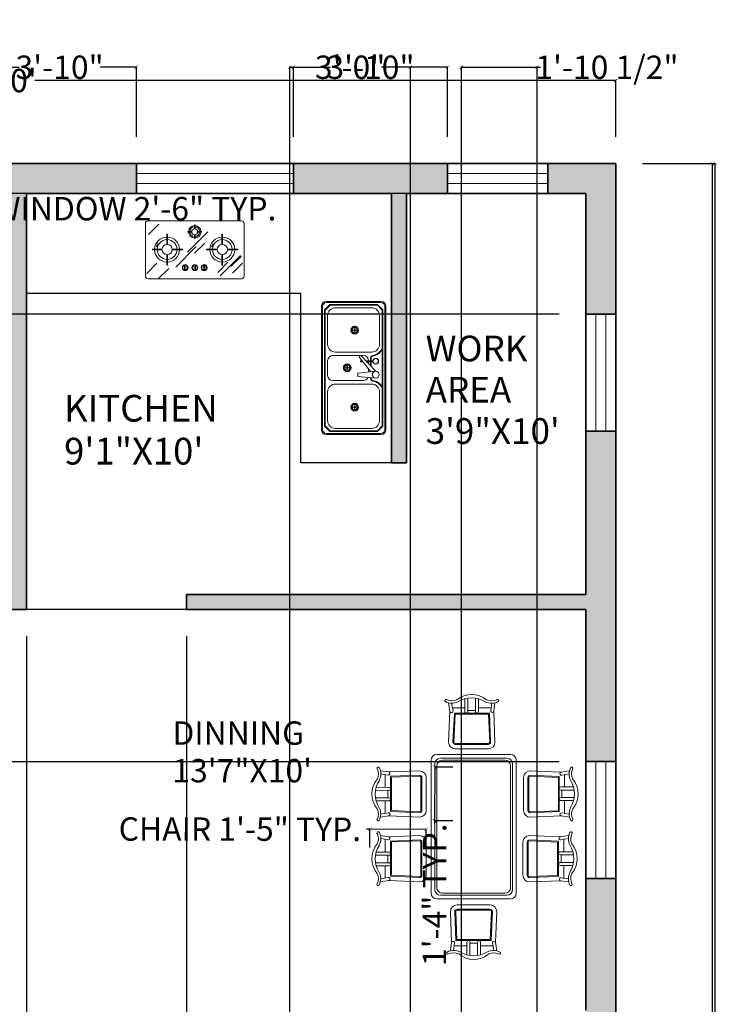
# Model space of a CAD drawing. Units: inches. Extents: x 98 to 545, y 56 to 703.
# Tile 4 of 4: x 324 to 537, y 408 to 703. Entities that reach past the tile are written whole.
import ezdxf

# ---------------------------------------------------------------- set-up
doc = ezdxf.new("R2010")
doc.units = ezdxf.units.IN
doc.header["$MEASUREMENT"] = 0
for name, color, linetype, lineweight in [('A-ANNO-DIMS', 2, 'Continuous', 18), ('A-AREA-IDEN', 7, 'Continuous', 25), ('A-EQPM', 8, 'Continuous', 15), ('A-FLOR-CASE', 8, 'Continuous', 25), ('A-FLOR-FIXT', 9, 'Continuous', 15), ('A-GLAZ', 4, 'Continuous', 18), ('A-WALL', 7, 'Continuous', 35), ('Furniture', 7, 'Continuous', 15)]:
    doc.layers.add(name, color=color, linetype=linetype, lineweight=lineweight)
doc.layers.add('A-WALL-PATT', color=18, linetype='Continuous', lineweight=13, true_color=0x000000)
doc.styles.get("Standard").update_dxf_attribs({"font": 'arial.ttf'})
doc.dimstyles.get("Standard").update_dxf_attribs({"dimtxt": 7, "dimasz": 1, "dimexe": 0.183, "dimexo": 8, "dimgap": 0.09, "dimtad": 0, "dimdec": 4, "dimzin": 0, "dimdsep": 46, "dimlunit": 3, "dimtxsty": 'Standard', "dimblk": 'ARCHTICK', "dimcen": 0, "dimclrd": 253, "dimclre": 251, "dimadec": 0, "dimazin": 0, "dimtfac": 1, "dimtdec": 4, "dimtofl": 0, "dimtmove": 0, "dimatfit": 3, "dimfxl": 1, "dimtolj": 1, "dimtzin": 0, "dimarcsym": 0})

# ---------------------------------------------------------------- blocks, each defined once
blk = doc.blocks.new('_ArchTick')
at = {"color": 0, "linetype": 'ByBlock', "const_width": 0.15}
blk.add_lwpolyline([(-0.5, -0.5), (0.5, 0.5)], dxfattribs=at)
blk = doc.blocks.new('*D2')
at = {"layer": 'A-ANNO-DIMS', "color": 0, "lineweight": -2, "transparency": 16777216}
for p, q in [((510.36, 659.7), (532.23, 659.7)), ((532.04, 659.7), (532.04, 395.87)), ((532.04, 119.7), (532.04, 383.53)), ((510.36, 119.7), (532.23, 119.7))]:
    blk.add_line(p, q, dxfattribs=at)
at = {"layer": 'Defpoints', "color": 0, "transparency": 16777216}
for p in [(502.36, 659.7), (502.36, 119.7), (532.04, 119.7)]:
    blk.add_point(p, dxfattribs=at)
at = {"layer": 'A-ANNO-DIMS', "color": 0, "lineweight": -2, "transparency": 16777216}
for p, rotation in [((532.04, 659.7), 90), ((532.04, 119.7), 270)]:
    blk.add_blockref('_ArchTick', p, dxfattribs=dict(at, rotation=rotation))
at = {"layer": 'A-ANNO-DIMS', "color": 0, "transparency": 16777216, "insert": (532.04, 389.7), "char_height": 7, "attachment_point": 5, "rotation": 90}
blk.add_mtext("\\A1;45'", dxfattribs=at)
blk = doc.blocks.new('*D4')
at = {"layer": 'A-ANNO-DIMS', "color": 0, "lineweight": -2, "transparency": 16777216}
for p, q in [((142.36, 667.7), (142.36, 684.75)), ((142.36, 684.57), (316.34, 684.57)), ((502.36, 684.57), (328.39, 684.57)), ((502.36, 667.7), (502.36, 684.75))]:
    blk.add_line(p, q, dxfattribs=at)
at = {"layer": 'Defpoints', "color": 0, "transparency": 16777216}
for p in [(502.36, 684.57), (142.36, 659.7), (502.36, 659.7)]:
    blk.add_point(p, dxfattribs=at)
at = {"layer": 'A-ANNO-DIMS', "color": 0, "lineweight": -2, "transparency": 16777216, "rotation": 180}
blk.add_blockref('_ArchTick', (142.36, 684.57), dxfattribs=at)
at = {"layer": 'A-ANNO-DIMS', "color": 0, "lineweight": -2, "transparency": 16777216}
blk.add_blockref('_ArchTick', (502.36, 684.57), dxfattribs=at)
at = {"layer": 'A-ANNO-DIMS', "color": 0, "transparency": 16777216, "insert": (322.36, 684.57), "char_height": 7, "attachment_point": 5}
blk.add_mtext("\\A1;30'", dxfattribs=at)
blk = doc.blocks.new('WIN-SASH-47IN')
for p, q in [((47, 9), (0, 9)), ((0, 6), (47, 6)), ((0, 3), (47, 3)), ((0, 0), (47, 0))]:
    blk.add_line(p, q)
blk = doc.blocks.new('WIN-SASH-35IN')
for p, q in [((0, 35), (0, 0)), ((3, 35), (3, 0)), ((6, 35), (6, 0)), ((9, 0), (9, 35))]:
    blk.add_line(p, q)
blk = doc.blocks.new('WIN-SASH-30IN')
for p, q in [((30, 9), (0, 9)), ((0, 6), (30, 6)), ((0, 3), (30, 3)), ((0, 0), (30, 0))]:
    blk.add_line(p, q)
blk = doc.blocks.new('CHAIR-DINING')
for p, q in [((1.98, 15), (11.17, 14.59)), ((11.17, 14.59), (13.72, 15)), ((0, 3.1), (0, 13.02)), ((1.3, 3.1), (1.3, 13.02)), ((1.59, 3.1), (1.59, 13.02)), ((1.98, 13.42), (10.39, 13.01)), ((2, 13.7), (10.68, 13.28)), ((10.39, 13.01), (10.39, 3.06)), ((10.68, 13.28), (10.68, 2.78)), ((11.39, 13.68), (13.6, 14.1)), ((12.26, 13.85), (12.26, 10.16)), ((11.22, 10.16), (14.96, 10.16)), ((11.22, 9.26), (15.16, 9.26)), ((11.47, 9.26), (11.47, 6.98)), ((15.16, 6.98), (11.22, 6.98)), ((14.97, 6.08), (11.23, 6.08)), ((12.26, 6.08), (12.26, 2.24)), ((10.39, 3.06), (1.98, 2.7)), ((11.24, 1.48), (1.98, 1.12)), ((10.68, 2.78), (2, 2.42)), ((13.72, 1.12), (11.24, 1.48)), ((13.6, 2.02), (11.39, 2.39))]:
    blk.add_line(p, q)
for centre, radius, start, end in [((1.98, 13.02), 1.98, 90, 180), ((17.59, 14.03), 3.98, 151.1173, 207.5141), ((14.4, 15.77), 0.355, 326.5726, 147.7215), ((17.59, 14.03), 3.28, 150.9211, 207.5141), ((1.98, 13.02), 0.68, 90, 180), ((1.98, 13.02), 0.397, 90, 180), ((11.28, 14.13), 0.467, 76.2748, 283.7252), ((7.66, 8.11), 7.58, 327.3186, 32.6814), ((9.31, 8.06), 6.98, 320.3459, 39.6541), ((11.13, 9.71), 0.463, 78.6748, 281.3252), ((11.13, 6.53), 0.463, 78.8014, 282.2085), ((1.98, 3.1), 1.98, 180, 270), ((1.98, 3.1), 0.68, 180, 270), ((1.98, 3.1), 0.397, 180, 270), ((17.59, 2.09), 3.98, 152.4859, 208.8827), ((17.59, 2.09), 3.28, 152.4859, 208.022), ((11.32, 1.93), 0.459, 80.8614, 279.1386), ((14.4, 0.36), 0.355, 212.2785, 33.4274)]:
    blk.add_arc(centre, radius, start, end)
blk = doc.blocks.new('*D13')
at = {"layer": 'A-ANNO-DIMS', "color": 253, "lineweight": -2, "transparency": 16777216}
for p, q in [((282.86, 646.2), (312.86, 646.2)), ((312.86, 646.2), (313.86, 646.2))]:
    blk.add_line(p, q, dxfattribs=at)
at = {"layer": 'A-ANNO-DIMS', "color": 251, "lineweight": -2, "transparency": 16777216}
for p, q in [((282.86, 642.7), (282.86, 646.01)), ((312.86, 642.7), (312.86, 646.01))]:
    blk.add_line(p, q, dxfattribs=at)
at = {"layer": 'Defpoints', "color": 0, "transparency": 16777216}
for p in [(282.86, 650.7), (312.86, 650.7), (312.86, 646.2)]:
    blk.add_point(p, dxfattribs=at)
at = {"layer": 'A-ANNO-DIMS', "color": 253, "lineweight": -2, "transparency": 16777216, "rotation": 180}
blk.add_blockref('_ArchTick', (282.86, 646.2), dxfattribs=at)
at = {"layer": 'A-ANNO-DIMS', "color": 253, "lineweight": -2, "transparency": 16777216}
blk.add_blockref('_ArchTick', (312.86, 646.2), dxfattribs=at)
at = {"layer": 'A-ANNO-DIMS', "color": 0, "transparency": 16777216, "insert": (358.24, 646.2), "char_height": 7, "attachment_point": 5}
blk.add_mtext('\\A1;WINDOW 2\'-6" TYP.', dxfattribs=at)
blk = doc.blocks.new('*D14')
at = {"layer": 'A-ANNO-DIMS', "color": 253, "lineweight": -2, "transparency": 16777216}
for p, q in [((317.36, 659.7), (317.36, 660.7)), ((317.36, 650.7), (317.36, 659.7))]:
    blk.add_line(p, q, dxfattribs=at)
at = {"layer": 'A-ANNO-DIMS', "color": 251, "lineweight": -2, "transparency": 16777216}
for p, q in [((320.86, 659.7), (317.55, 659.7)), ((320.86, 650.7), (317.55, 650.7))]:
    blk.add_line(p, q, dxfattribs=at)
at = {"layer": 'Defpoints', "color": 0, "transparency": 16777216}
for p in [(312.86, 659.7), (317.36, 659.7), (312.86, 650.7)]:
    blk.add_point(p, dxfattribs=at)
at = {"layer": 'A-ANNO-DIMS', "color": 253, "lineweight": -2, "transparency": 16777216}
for p, rotation in [((317.36, 659.7), 90), ((317.36, 650.7), 270)]:
    blk.add_blockref('_ArchTick', p, dxfattribs=dict(at, rotation=rotation))
at = {"layer": 'A-ANNO-DIMS', "color": 0, "transparency": 16777216, "insert": (317.36, 682.12), "char_height": 7, "attachment_point": 5, "rotation": 90}
blk.add_mtext('\\A1;0\'-9" TYP.', dxfattribs=at)
blk = doc.blocks.new('*D15')
at = {"layer": 'A-ANNO-DIMS', "color": 253, "lineweight": -2, "transparency": 16777216}
for p, q in [((428.76, 460.37), (427.76, 460.37)), ((445.58, 460.35), (428.76, 460.37))]:
    blk.add_line(p, q, dxfattribs=at)
at = {"layer": 'A-ANNO-DIMS', "color": 251, "lineweight": -2, "transparency": 16777216}
for p, q in [((428.75, 454.89), (428.76, 460.19)), ((445.58, 454.87), (445.58, 460.17))]:
    blk.add_line(p, q, dxfattribs=at)
at = {"layer": 'Defpoints', "color": 0, "transparency": 16777216}
for p in [(428.76, 462.89), (445.59, 462.87), (428.76, 460.37)]:
    blk.add_point(p, dxfattribs=at)
at = {"layer": 'A-ANNO-DIMS', "color": 253, "lineweight": -2, "transparency": 16777216}
for p, rotation in [((428.76, 460.37), 179.9304565609884), ((445.58, 460.35), 359.9304565609884)]:
    blk.add_blockref('_ArchTick', p, dxfattribs=dict(at, rotation=rotation))
at = {"layer": 'A-ANNO-DIMS', "color": 0, "transparency": 16777216, "insert": (389.8, 460.42), "char_height": 7, "attachment_point": 5, "rotation": 359.9305}
blk.add_mtext('\\A1;CHAIR 1\'-5" TYP.', dxfattribs=at)
blk = doc.blocks.new('*D16')
at = {"layer": 'A-ANNO-DIMS', "color": 253, "lineweight": -2, "transparency": 16777216}
for p, q in [((448.13, 479), (448.11, 462.87)), ((448.11, 462.87), (448.11, 461.87))]:
    blk.add_line(p, q, dxfattribs=at)
at = {"layer": 'A-ANNO-DIMS', "color": 251, "lineweight": -2, "transparency": 16777216}
for p, q in [((453.61, 479), (448.31, 479)), ((453.59, 462.86), (448.29, 462.87))]:
    blk.add_line(p, q, dxfattribs=at)
at = {"layer": 'Defpoints', "color": 0, "transparency": 16777216}
for p in [(445.61, 479.01), (445.59, 462.87), (448.11, 462.87)]:
    blk.add_point(p, dxfattribs=at)
at = {"layer": 'A-ANNO-DIMS', "color": 253, "lineweight": -2, "transparency": 16777216}
for p, rotation in [((448.13, 479), 89.93045656098832), ((448.11, 462.87), 269.9304565609883)]:
    blk.add_blockref('_ArchTick', p, dxfattribs=dict(at, rotation=rotation))
at = {"layer": 'A-ANNO-DIMS', "color": 0, "transparency": 16777216, "insert": (448.08, 440.78), "char_height": 7, "attachment_point": 5, "rotation": 89.9305}
blk.add_mtext('\\A1;1\'-4" TYP.', dxfattribs=at)
blk = doc.blocks.new('*D17')
at = {"layer": 'A-ANNO-DIMS', "color": 251, "lineweight": -2, "transparency": 16777216}
for p, q in [((510.36, 659.7), (531.4, 659.7)), ((446.43, 95.7), (531.4, 95.7))]:
    blk.add_line(p, q, dxfattribs=at)
at = {"layer": 'A-ANNO-DIMS', "color": 253, "lineweight": -2, "transparency": 16777216}
for p, q in [((531.21, 659.7), (531.21, 389.95)), ((531.21, 95.7), (531.21, 365.44))]:
    blk.add_line(p, q, dxfattribs=at)
at = {"layer": 'Defpoints', "color": 0, "transparency": 16777216}
for p in [(502.36, 659.7), (531.21, 659.7), (438.43, 95.7)]:
    blk.add_point(p, dxfattribs=at)
at = {"layer": 'A-ANNO-DIMS', "color": 253, "lineweight": -2, "transparency": 16777216}
for p, rotation in [((531.21, 659.7), 90), ((531.21, 95.7), 270)]:
    blk.add_blockref('_ArchTick', p, dxfattribs=dict(at, rotation=rotation))
at = {"layer": 'A-ANNO-DIMS', "color": 0, "transparency": 16777216, "insert": (531.21, 377.7), "char_height": 7, "attachment_point": 5, "rotation": 90}
blk.add_mtext('\\A1;47\'-0"', dxfattribs=at)
blk = doc.blocks.new('*D23')
at = {"layer": 'A-ANNO-DIMS', "color": 251, "lineweight": -2, "transparency": 16777216}
for p, q in [((312.86, 667.7), (312.86, 688.73)), ((358.82, 667.7), (358.82, 688.73))]:
    blk.add_line(p, q, dxfattribs=at)
at = {"layer": 'A-ANNO-DIMS', "color": 253, "lineweight": -2, "transparency": 16777216}
for p, q in [((312.86, 688.55), (323.73, 688.55)), ((358.82, 688.55), (347.95, 688.55))]:
    blk.add_line(p, q, dxfattribs=at)
at = {"layer": 'Defpoints', "color": 0, "transparency": 16777216}
for p in [(358.82, 688.55), (312.86, 659.7), (358.82, 659.7)]:
    blk.add_point(p, dxfattribs=at)
at = {"layer": 'A-ANNO-DIMS', "color": 253, "lineweight": -2, "transparency": 16777216, "rotation": 180}
blk.add_blockref('_ArchTick', (312.86, 688.55), dxfattribs=at)
at = {"layer": 'A-ANNO-DIMS', "color": 253, "lineweight": -2, "transparency": 16777216}
blk.add_blockref('_ArchTick', (358.82, 688.55), dxfattribs=at)
at = {"layer": 'A-ANNO-DIMS', "color": 0, "transparency": 16777216, "insert": (335.84, 688.55), "char_height": 7, "attachment_point": 5}
blk.add_mtext('\\A1;3\'-10"', dxfattribs=at)
blk = doc.blocks.new('*D24')
at = {"layer": 'A-ANNO-DIMS', "color": 251, "lineweight": -2, "transparency": 16777216}
for p, q in [((405.82, 667.7), (405.82, 688.73)), ((451.99, 667.7), (451.99, 688.73))]:
    blk.add_line(p, q, dxfattribs=at)
at = {"layer": 'A-ANNO-DIMS', "color": 253, "lineweight": -2, "transparency": 16777216}
for p, q in [((405.82, 688.55), (416.79, 688.55)), ((451.99, 688.55), (441.02, 688.55))]:
    blk.add_line(p, q, dxfattribs=at)
at = {"layer": 'Defpoints', "color": 0, "transparency": 16777216}
for p in [(451.99, 688.55), (405.82, 659.7), (451.99, 659.7)]:
    blk.add_point(p, dxfattribs=at)
at = {"layer": 'A-ANNO-DIMS', "color": 253, "lineweight": -2, "transparency": 16777216, "rotation": 180}
blk.add_blockref('_ArchTick', (405.82, 688.55), dxfattribs=at)
at = {"layer": 'A-ANNO-DIMS', "color": 253, "lineweight": -2, "transparency": 16777216}
blk.add_blockref('_ArchTick', (451.99, 688.55), dxfattribs=at)
at = {"layer": 'A-ANNO-DIMS', "color": 0, "transparency": 16777216, "insert": (428.91, 688.55), "char_height": 7, "attachment_point": 5}
blk.add_mtext('\\A1;3\'-10"', dxfattribs=at)
blk = doc.blocks.new('*D31')
at = {"layer": 'A-ANNO-DIMS', "color": 251, "lineweight": -2, "transparency": 16777216}
for p, q in [((485.36, 650.7), (113.33, 650.7)), ((485.36, 614.58), (113.33, 614.58))]:
    blk.add_line(p, q, dxfattribs=at)
at = {"layer": 'A-ANNO-DIMS', "color": 253, "lineweight": -2, "transparency": 16777216}
for p, q in [((113.51, 650.7), (113.51, 642.03)), ((113.51, 614.58), (113.51, 623.25))]:
    blk.add_line(p, q, dxfattribs=at)
at = {"layer": 'Defpoints', "color": 0, "transparency": 16777216}
for p in [(493.36, 650.7), (113.51, 614.58), (493.36, 614.58)]:
    blk.add_point(p, dxfattribs=at)
at = {"layer": 'A-ANNO-DIMS', "color": 253, "lineweight": -2, "transparency": 16777216}
for p, rotation in [((113.51, 650.7), 90), ((113.51, 614.58), 270)]:
    blk.add_blockref('_ArchTick', p, dxfattribs=dict(at, rotation=rotation))
at = {"layer": 'A-ANNO-DIMS', "color": 0, "transparency": 16777216, "insert": (113.51, 632.64), "char_height": 7, "attachment_point": 5, "rotation": 90}
blk.add_mtext('\\A1;3\'-0"', dxfattribs=at)
blk = doc.blocks.new('*D32')
at = {"layer": 'A-ANNO-DIMS', "color": 251, "lineweight": -2, "transparency": 16777216}
for p, q in [((485.36, 526.2), (113.33, 526.2)), ((485.36, 480.62), (113.33, 480.62))]:
    blk.add_line(p, q, dxfattribs=at)
at = {"layer": 'A-ANNO-DIMS', "color": 253, "lineweight": -2, "transparency": 16777216}
for p, q in [((113.51, 526.2), (113.51, 520.96)), ((113.51, 480.62), (113.51, 485.86))]:
    blk.add_line(p, q, dxfattribs=at)
at = {"layer": 'Defpoints', "color": 0, "transparency": 16777216}
for p in [(493.36, 526.2), (113.51, 480.62), (493.36, 480.62)]:
    blk.add_point(p, dxfattribs=at)
at = {"layer": 'A-ANNO-DIMS', "color": 253, "lineweight": -2, "transparency": 16777216}
for p, rotation in [((113.51, 526.2), 90), ((113.51, 480.62), 270)]:
    blk.add_blockref('_ArchTick', p, dxfattribs=dict(at, rotation=rotation))
at = {"layer": 'A-ANNO-DIMS', "color": 0, "transparency": 16777216, "insert": (113.51, 503.41), "char_height": 7, "attachment_point": 5, "rotation": 90}
blk.add_mtext('\\A1;3\'-9 1/2"', dxfattribs=at)
blk = doc.blocks.new('*D34')
at = {"layer": 'A-ANNO-DIMS', "color": 251, "lineweight": -2, "transparency": 16777216}
for p, q in [((404.75, 201.2), (404.75, 688.73)), ((440.86, 201.2), (440.86, 688.73))]:
    blk.add_line(p, q, dxfattribs=at)
at = {"layer": 'A-ANNO-DIMS', "color": 253, "lineweight": -2, "transparency": 16777216}
for p, q in [((404.75, 688.55), (413.41, 688.55)), ((440.86, 688.55), (432.2, 688.55))]:
    blk.add_line(p, q, dxfattribs=at)
at = {"layer": 'Defpoints', "color": 0, "transparency": 16777216}
for p in [(440.86, 688.55), (404.75, 193.2), (440.86, 193.2)]:
    blk.add_point(p, dxfattribs=at)
at = {"layer": 'A-ANNO-DIMS', "color": 253, "lineweight": -2, "transparency": 16777216, "rotation": 180}
blk.add_blockref('_ArchTick', (404.75, 688.55), dxfattribs=at)
at = {"layer": 'A-ANNO-DIMS', "color": 253, "lineweight": -2, "transparency": 16777216}
blk.add_blockref('_ArchTick', (440.86, 688.55), dxfattribs=at)
at = {"layer": 'A-ANNO-DIMS', "color": 0, "transparency": 16777216, "insert": (422.81, 688.55), "char_height": 7, "attachment_point": 5}
blk.add_mtext('\\A1;3\'-0"', dxfattribs=at)
blk = doc.blocks.new('*D35')
at = {"layer": 'A-ANNO-DIMS', "color": 251, "lineweight": -2, "transparency": 16777216}
for p, q in [((456.13, 201.2), (456.13, 688.73)), ((478.77, 201.2), (478.77, 688.73))]:
    blk.add_line(p, q, dxfattribs=at)
at = {"layer": 'A-ANNO-DIMS', "color": 253, "lineweight": -2, "transparency": 16777216}
for p, q in [((456.13, 688.55), (478.77, 688.55)), ((478.77, 688.55), (479.77, 688.55))]:
    blk.add_line(p, q, dxfattribs=at)
at = {"layer": 'Defpoints', "color": 0, "transparency": 16777216}
for p in [(478.77, 688.55), (456.13, 193.2), (478.77, 193.2)]:
    blk.add_point(p, dxfattribs=at)
at = {"layer": 'A-ANNO-DIMS', "color": 253, "lineweight": -2, "transparency": 16777216, "rotation": 180}
blk.add_blockref('_ArchTick', (456.13, 688.55), dxfattribs=at)
at = {"layer": 'A-ANNO-DIMS', "color": 253, "lineweight": -2, "transparency": 16777216}
blk.add_blockref('_ArchTick', (478.77, 688.55), dxfattribs=at)
at = {"layer": 'A-ANNO-DIMS', "color": 0, "transparency": 16777216, "insert": (499.7, 688.55), "char_height": 7, "attachment_point": 5}
blk.add_mtext('\\A1;1\'-10 1/2"', dxfattribs=at)
blk = doc.blocks.new('*D36')
at = {"layer": 'A-ANNO-DIMS', "color": 251, "lineweight": -2, "transparency": 16777216}
for p, q in [((325.96, 518.2), (325.96, 66.66)), ((373.81, 518.2), (373.81, 66.66))]:
    blk.add_line(p, q, dxfattribs=at)
at = {"layer": 'A-ANNO-DIMS', "color": 253, "lineweight": -2, "transparency": 16777216}
for p, q in [((325.96, 66.85), (340.35, 66.85)), ((373.81, 66.85), (359.42, 66.85))]:
    blk.add_line(p, q, dxfattribs=at)
at = {"layer": 'Defpoints', "color": 0, "transparency": 16777216}
for p in [(325.96, 526.2), (373.81, 526.2), (373.81, 66.85)]:
    blk.add_point(p, dxfattribs=at)
at = {"layer": 'A-ANNO-DIMS', "color": 253, "lineweight": -2, "transparency": 16777216, "rotation": 180}
blk.add_blockref('_ArchTick', (325.96, 66.85), dxfattribs=at)
at = {"layer": 'A-ANNO-DIMS', "color": 253, "lineweight": -2, "transparency": 16777216}
blk.add_blockref('_ArchTick', (373.81, 66.85), dxfattribs=at)
at = {"layer": 'A-ANNO-DIMS', "color": 0, "transparency": 16777216, "insert": (349.89, 66.85), "char_height": 7, "attachment_point": 5}
blk.add_mtext('\\A1;4\'-0"', dxfattribs=at)

msp = doc.modelspace()

# ---------------------------------------------------------------- hatches: boundary and pattern name
at = {"layer": 'A-WALL-PATT'}
h = msp.add_hatch(color=256, dxfattribs=at)
h.dxf.hatch_style = 1
h.paths.add_polyline_path([(173.39577, 659.69681), (142.36469, 659.69681), (142.36469, 612.44216), (151.36469, 612.44216), (151.36469, 650.69681), (173.39577, 650.69681)])
h.paths.add_polyline_path([(282.86266, 659.69681), (220.39577, 659.69681), (220.39577, 650.69681), (271.36469, 650.69681), (271.36469, 566.19681), (275.86469, 566.19681), (288.55623, 566.19681), (288.55623, 570.69681), (275.86469, 570.69681), (275.86469, 650.69681), (282.86266, 650.69681)])
h.paths.add_polyline_path([(358.82163, 659.69681), (312.86266, 659.69681), (312.86266, 650.69681), (321.46469, 650.69681), (321.46469, 570.69681), (321.46469, 566.19681), (321.46469, 530.69681), (321.46469, 526.19681), (325.96469, 526.19681), (325.96469, 530.69681), (325.96469, 650.69681), (358.82163, 650.69681)])
h.paths.add_polyline_path([(451.98971, 659.69681), (405.82163, 659.69681), (405.82163, 650.69681), (435.16469, 650.69681), (435.16469, 570.08746), (439.66469, 570.08746), (439.66469, 650.69681), (451.98971, 650.69681)])
h.paths.add_polyline_path([(502.36469, 659.69681), (481.98971, 659.69681), (481.98971, 650.69681), (493.36469, 650.69681), (493.36469, 614.57752), (502.36469, 614.57752)])
h.paths.add_polyline_path([(502.36469, 579.57752), (493.36469, 579.57752), (493.36469, 530.69681), (439.66469, 530.69681), (435.16469, 530.69681), (373.81242, 530.69681), (373.81242, 526.19681), (493.36469, 526.19681), (493.36469, 480.62471), (502.36469, 480.62471)])
h.paths.add_polyline_path([(502.36469, 445.62471), (493.36469, 445.62471), (493.36469, 406.19681), (493.36469, 401.69681), (493.36469, 397.69681), (379.47742, 397.69681), (379.47742, 393.19681), (493.36469, 393.19681), (493.36469, 306.38501), (502.36469, 306.38501)])
h.paths.add_polyline_path([(502.36469, 271.38501), (493.36469, 271.38501), (493.36469, 193.19681), (478.76571, 193.19681), (478.76571, 188.69681), (493.36469, 188.69681), (493.36469, 128.69681), (487.75103, 128.69681), (487.75103, 119.69681), (502.36469, 119.69681)])
h.paths.add_polyline_path([(452.75103, 128.69681), (445.36469, 128.69681), (445.36469, 188.69681), (456.12508, 188.69681), (456.12508, 193.19681), (440.86469, 193.19681), (440.86469, 119.69681), (452.75103, 119.69681)])
h.paths.add_polyline_path([(307.21941, 128.69681), (293.86469, 128.69681), (293.86469, 188.69681), (404.74827, 188.69681), (404.74827, 193.19681), (293.86469, 193.19681), (293.86469, 306.29681), (289.36469, 306.29681), (289.36469, 119.69681), (307.21941, 119.69681)])
h.paths.add_polyline_path([(289.36469, 161.69681), (238.02122, 161.69681), (238.02122, 152.69681), (289.36469, 152.69681)])
h.paths.add_polyline_path([(191.02122, 161.69681), (151.36469, 161.69681), (151.36469, 191.65928), (142.36469, 191.65928), (142.36469, 152.69681), (151.36469, 152.69681), (191.02122, 152.69681)])
h.paths.add_polyline_path([(151.36469, 306.29681), (151.36469, 308.54862), (142.36469, 308.54862), (142.36469, 238.65928), (151.36469, 238.65928)])
h.paths.add_polyline_path([(230.26469, 401.69681), (230.26469, 406.19681), (182.81458, 406.19681), (182.81458, 401.69681), (225.76469, 401.69681), (225.76469, 358.49681), (151.36469, 358.49681), (151.36469, 368.55378), (142.36469, 368.55378), (142.36469, 338.54862), (151.36469, 338.54862), (151.36469, 353.99681), (225.76469, 353.99681), (225.76469, 310.79681), (180.84919, 310.79681), (180.84919, 306.29681), (230.26469, 306.29681)])
h.paths.add_polyline_path([(151.36469, 442.07867), (142.36469, 442.07867), (142.36469, 398.55378), (151.36469, 398.55378), (151.36469, 401.69681)])
h.paths.add_polyline_path([(151.36469, 526.19681), (271.36469, 526.19681), (271.36469, 406.19681), (271.36469, 401.69681), (275.86469, 401.69681), (275.86469, 406.19681), (275.86469, 526.19681), (275.86469, 530.69681), (271.36469, 530.69681), (151.36469, 530.69681), (151.36469, 565.44216), (142.36469, 565.44216), (142.36469, 489.07867), (151.36469, 489.07867)])

# ---------------------------------------------------------------- linework, layer by layer
at = {"layer": 'A-EQPM'}
for p, q in [((361.51272, 641.75689), (361.51272, 626.00889)), ((390.25282, 642.54429), (362.30012, 642.54429)), ((362.45426, 638.48), (365.50107, 641.52681)), ((376.17804, 640.36597), (376.17804, 641.38815)), ((376.37489, 641.38815), (376.17804, 641.38815)), ((376.37489, 640.36597), (376.37489, 641.38815)), ((391.04022, 626.00889), (391.04022, 641.75689)), ((367.91333, 638.60488), (368.11018, 638.60488)), ((367.91333, 635.73909), (367.91333, 638.60488)), ((368.11018, 635.73909), (368.11018, 638.60488)), ((374.14768, 633.2007), (380.2413, 639.29432)), ((375.19908, 639.387), (374.20116, 639.387)), ((374.20116, 639.19015), (374.20116, 639.387)), ((375.19908, 639.19015), (374.20116, 639.19015)), ((376.17804, 638.21119), (376.17804, 637.25312)), ((376.37489, 637.25312), (376.17804, 637.25312)), ((376.37489, 638.21119), (376.37489, 637.25312)), ((377.35386, 639.387), (378.32775, 639.387)), ((377.35386, 639.19015), (378.32775, 639.19015)), ((378.32775, 639.387), (378.32775, 639.19015)), ((384.63961, 638.60488), (384.44276, 638.60488)), ((384.44276, 635.73909), (384.44276, 638.60488)), ((384.63961, 635.73909), (384.63961, 638.60488)), ((363.60605, 634.0686), (363.60605, 633.87175)), ((366.24284, 634.0686), (363.60605, 634.0686)), ((366.24284, 633.87175), (363.60605, 633.87175)), ((369.78067, 634.0686), (372.693, 634.0686)), ((369.78067, 633.87175), (372.693, 633.87175)), ((370.65131, 628.73658), (376.74493, 634.8302)), ((372.693, 634.0686), (372.693, 633.87175)), ((376.2455, 632.85133), (379.29232, 635.89814)), ((379.85993, 634.0686), (379.85993, 633.87175)), ((382.77227, 634.0686), (379.85993, 634.0686)), ((382.77227, 633.87175), (379.85993, 633.87175)), ((386.3101, 634.0686), (389.14374, 634.0686)), ((386.3101, 633.87175), (389.14374, 633.87175)), ((389.14374, 634.0686), (389.14374, 633.87175)), ((367.91333, 632.20126), (367.91333, 629.30549)), ((368.11018, 632.20126), (368.11018, 629.30549)), ((383.85983, 626.09693), (389.95345, 632.19055)), ((384.44276, 632.20126), (384.44276, 629.30549)), ((384.63961, 632.20126), (384.63961, 629.30549)), ((387.12311, 628.85028), (390.16992, 631.89709)), ((361.91038, 626.83448), (364.95719, 629.88129)), ((365.48445, 625.28175), (368.53126, 628.32856)), ((367.91333, 629.30549), (368.11018, 629.30549)), ((373.27026, 629.1496), (373.27026, 627.93933)), ((373.58522, 629.1496), (373.58522, 627.93933)), ((376.15766, 629.1496), (376.15766, 627.93933)), ((376.47262, 629.1496), (376.47262, 627.93933)), ((378.96772, 629.1496), (378.96772, 627.93933)), ((379.28268, 629.1496), (379.28268, 627.93933)), ((383.16055, 627.10621), (386.20736, 630.15302)), ((384.63961, 629.30549), (384.44276, 629.30549)), ((387.55044, 626.8733), (390.59725, 629.92011)), ((362.30012, 625.22149), (390.25282, 625.22149))]:
    msp.add_line(p, q, dxfattribs=at)
for centre, radius in [((375.13175, 640.42965), 0.14703), ((376.27647, 639.28858), 0.88054), ((365.02178, 634.99687), 0.14703), ((365.24037, 635.51558), 0.14703), ((368.01176, 633.97018), 1.53543), ((381.55294, 634.96957), 0.14703), ((381.77154, 635.48828), 0.14703), ((384.54118, 633.97018), 1.53543), ((373.42774, 628.54447), 0.88583), ((376.31514, 628.54447), 0.88583), ((379.1252, 628.54447), 0.88583)]:
    msp.add_circle(centre, radius, dxfattribs=at)
for centre, radius, start, end in [((362.30012, 641.75689), 0.7874, 90, 180), ((376.27647, 639.28858), 1.86479, 93.0255225, 176.9744775), ((376.27647, 639.28858), 1.47109, 93.8363117, 176.1636883), ((376.27647, 640.37971), 0.09938, 187.9505325, 352.0494675), ((376.27647, 639.28858), 1.86479, 3.0255225, 86.9744775), ((376.27647, 639.28858), 1.47109, 3.8363117, 86.1636883), ((390.25282, 641.75689), 0.7874, 0, 90), ((368.01176, 633.97018), 3.74015, 91.5917542, 178.4082458), ((368.01176, 633.97018), 2.95275, 91.9102132, 178.0897868), ((368.01176, 633.97018), 2.95275, 1.9102132, 88.0897868), ((368.01176, 633.97018), 3.74015, 1.5917542, 88.4082458), ((376.27647, 639.28858), 1.86479, 183.0255225, 266.9744775), ((376.27647, 639.28858), 1.47109, 183.8363117, 266.1636883), ((375.1678, 639.28858), 0.10328, 287.6317755, 72.3682245), ((376.27647, 638.21406), 0.09847, 358.3317253, 181.6682747), ((376.27647, 639.28858), 1.47109, 273.8363117, 356.1636883), ((376.27647, 639.28858), 1.86479, 273.0255225, 356.9744775), ((377.36633, 639.28858), 0.09921, 97.2236134, 262.7763866), ((384.54118, 633.97018), 3.74015, 91.5917542, 178.4082458), ((384.54118, 633.97018), 2.95275, 91.9102132, 178.0897868), ((384.54118, 633.97018), 2.95275, 1.9102132, 88.0897868), ((384.54118, 633.97018), 3.74015, 1.5917542, 88.4082458), ((368.01176, 633.97018), 3.74015, 181.5917542, 268.4082458), ((368.01176, 633.97018), 2.95275, 181.9102132, 268.0897868), ((366.20943, 633.97018), 0.10394, 288.751046, 71.248954), ((368.01176, 635.75072), 0.09911, 186.7353744, 353.2646256), ((368.01176, 633.97018), 2.95275, 271.9102132, 358.0897868), ((368.01176, 633.97018), 3.74015, 271.5917542, 358.4082458), ((369.81757, 633.97018), 0.10511, 110.550693, 249.449307), ((384.54118, 633.97018), 3.74015, 181.5917542, 268.4082458), ((384.54118, 633.97018), 2.95275, 181.9102132, 268.0897868), ((382.7395, 633.97018), 0.10374, 288.4119714, 71.5880286), ((384.54118, 635.7459), 0.09866, 183.9579348, 356.0420652), ((384.54118, 633.97018), 2.95275, 271.9102132, 358.0897868), ((384.54118, 633.97018), 3.74015, 271.5917542, 358.4082458), ((386.33517, 633.97018), 0.10157, 104.2944789, 255.7055211), ((368.01176, 632.16192), 0.106, 21.7885229, 158.2114771), ((384.54118, 632.16939), 0.10346, 17.9418038, 162.0581962), ((373.42774, 628.54447), 0.72835, 111.3236863, 248.6763137), ((373.19152, 629.1496), 0.07874, 0, 111.3236863), ((373.66396, 629.1496), 0.07874, 68.6763137, 180), ((373.42774, 628.54447), 0.72835, 291.3236863, 68.6763137), ((376.31514, 628.54447), 0.72835, 111.3236863, 248.6763137), ((376.07892, 629.1496), 0.07874, 0, 111.3236863), ((376.55136, 629.1496), 0.07874, 68.6763137, 180), ((376.31514, 628.54447), 0.72835, 291.3236863, 68.6763137), ((379.1252, 628.54447), 0.72835, 111.3236863, 248.6763137), ((378.88898, 629.1496), 0.07874, 0, 111.3236863), ((379.36142, 629.1496), 0.07874, 68.6763137, 180), ((379.1252, 628.54447), 0.72835, 291.3236863, 68.6763137), ((362.30012, 626.00889), 0.7874, 180, 270), ((373.19152, 627.93933), 0.07874, 248.6763137, 0), ((373.66396, 627.93933), 0.07874, 180, 291.3236863), ((376.07892, 627.93933), 0.07874, 248.6763137, 0), ((376.55136, 627.93933), 0.07874, 180, 291.3236863), ((378.88898, 627.93933), 0.07874, 248.6763137, 0), ((379.36142, 627.93933), 0.07874, 180, 291.3236863), ((390.25282, 626.00889), 0.7874, 270, 360)]:
    msp.add_arc(centre, radius, start, end, dxfattribs=at)
at = {"layer": 'A-FLOR-CASE'}
for p, q in [((408.05328, 620.79618), (325.96469, 620.79618)), ((408.05328, 570.08746), (408.05328, 620.79618)), ((435.16469, 570.08746), (408.05328, 570.08746))]:
    msp.add_line(p, q, dxfattribs=at)
at = {"layer": 'A-FLOR-FIXT'}
for p, q in [((414.24106, 616.9979), (414.24106, 579.9901)), ((414.55602, 616.87979), (414.55602, 580.10821)), ((416.72137, 617.47034), (415.14657, 615.89554)), ((416.80291, 617.27349), (415.34342, 615.81401)), ((432.15441, 618.37585), (415.61901, 618.37585)), ((432.0363, 618.06089), (415.73712, 618.06089)), ((431.05205, 617.47034), (416.72137, 617.47034)), ((430.97051, 617.27349), (416.80291, 617.27349)), ((429.27906, 616.54375), (418.43536, 616.54375)), ((432.43, 615.81401), (430.97051, 617.27349)), ((432.62685, 615.89554), (431.05205, 617.47034)), ((433.2174, 580.10821), (433.2174, 616.87979)), ((433.53236, 579.9901), (433.53236, 616.9979)), ((415.14657, 615.89554), (415.14657, 581.09246)), ((415.34342, 615.81401), (415.34342, 581.174)), ((416.07316, 614.18155), (416.07316, 605.6058)), ((431.64126, 605.6058), (431.64126, 614.18155)), ((432.43, 604.54879), (432.43, 615.81401)), ((432.62685, 581.09246), (432.62685, 615.89554)), ((424.19732, 610.01737), (424.19732, 610.60787)), ((423.99345, 609.8135), (423.40295, 609.8135)), ((424.19732, 609.60964), (424.19732, 609.01914)), ((424.40118, 609.8135), (424.99168, 609.8135)), ((426.78239, 602.24116), (417.65026, 602.24116)), ((418.43536, 603.2436), (429.27906, 603.2436)), ((429.01355, 597.37003), (425.64538, 601.67341)), ((425.69408, 602.1114), (425.71792, 602.13088)), ((430.4927, 597.53283), (426.14548, 602.10407)), ((428.91412, 600.61734), (428.91412, 601.50269)), ((429.11097, 600.61734), (429.11097, 601.50269)), ((432.43, 592.77619), (432.43, 604.08718)), ((416.07546, 600.66636), (416.07546, 596.30984)), ((421.74556, 598.56586), (421.15506, 598.56586)), ((421.94943, 598.76973), (421.94943, 599.36023)), ((422.1533, 598.56586), (422.7438, 598.56586)), ((425.93131, 600.37108), (425.93131, 600.61734)), ((425.93131, 600.61734), (426.47195, 600.61734)), ((426.66469, 600.37108), (425.93131, 600.37108)), ((427.55934, 600.61734), (429.61935, 600.61734)), ((429.62517, 600.37108), (427.79353, 600.37108)), ((428.35719, 600.61734), (428.35719, 600.66636)), ((428.35719, 599.77838), (428.35719, 600.37108)), ((428.91412, 599.19275), (428.91412, 600.37108)), ((429.11097, 598.98576), (429.11097, 600.37108)), ((421.94943, 598.36199), (421.94943, 597.7715)), ((425.08836, 596.7618), (425.08791, 596.19526)), ((430.4927, 597.53283), (425.26368, 596.95731)), ((425.26531, 595.99922), (430.4927, 595.48017)), ((428.35719, 597.29779), (428.35719, 598.20863)), ((428.91412, 597.35909), (428.91412, 597.49706)), ((428.91412, 595.36068), (428.91412, 595.63691)), ((429.11097, 595.36068), (429.11097, 595.61737)), ((417.65026, 594.73504), (426.78239, 594.73504)), ((429.27906, 593.69698), (418.43536, 593.69698)), ((416.07316, 591.33478), (416.07316, 582.75903)), ((431.64126, 582.75903), (431.64126, 591.33478)), ((432.43, 581.174), (432.43, 592.31458)), ((423.99345, 586.75584), (423.40295, 586.75584)), ((424.19732, 586.95971), (424.19732, 587.55021)), ((424.40118, 586.75584), (424.99168, 586.75584)), ((424.19732, 586.55197), (424.19732, 585.96147)), ((415.14657, 581.09246), (416.72137, 579.51766)), ((415.34342, 581.174), (416.80291, 579.71451)), ((430.97051, 579.71451), (432.43, 581.174)), ((431.05205, 579.51766), (432.62685, 581.09246)), ((415.61901, 578.61215), (432.15441, 578.61215)), ((415.73712, 578.92711), (432.0363, 578.92711)), ((416.72137, 579.51766), (431.05205, 579.51766)), ((416.80291, 579.71451), (430.97051, 579.71451)), ((418.43536, 580.39683), (429.27906, 580.39683))]:
    msp.add_line(p, q, dxfattribs=at)
for centre, radius in [((424.19732, 609.8135), 1.16204), ((424.19732, 609.8135), 1.09933), ((424.19732, 609.8135), 0.83003), ((424.19732, 609.8135), 0.79437), ((424.19732, 609.8135), 0.20387), ((424.19732, 609.8135), 0.09579), ((421.94943, 598.56586), 1.16204), ((421.94943, 598.56586), 1.09933), ((421.94943, 598.56586), 0.83003), ((421.94943, 598.56586), 0.79437), ((421.94943, 598.56586), 0.20387), ((421.94943, 598.56586), 0.09579), ((430.47936, 600.51447), 0.86614), ((430.47936, 600.51447), 0.7874), ((430.4927, 596.5065), 1.02633), ((424.19732, 586.75584), 1.16204), ((424.19732, 586.75584), 1.09933), ((424.19732, 586.75584), 0.83003), ((424.19732, 586.75584), 0.79437), ((424.19732, 586.75584), 0.20387), ((424.19732, 586.75584), 0.09579)]:
    msp.add_circle(centre, radius, dxfattribs=at)
for centre, radius, start, end in [((415.61901, 616.9979), 1.37795, 90, 180), ((415.73712, 616.87979), 1.1811, 90, 180), ((418.43536, 614.18155), 2.3622, 90, 180), ((429.27906, 614.18155), 2.3622, 0, 90), ((432.0363, 616.87979), 1.1811, 0, 90), ((432.15441, 616.9979), 1.37795, 0, 90), ((418.43536, 605.6058), 2.3622, 180, 270), ((429.27906, 605.6058), 2.3622, 270, 0), ((428.99493, 605.94046), 3.70627, 279.0468295, 337.9454022), ((417.65026, 600.66636), 1.5748, 90, 180), ((425.89341, 601.86754), 0.31496, 129.2618707, 218.0494843), ((425.91724, 601.88702), 0.31496, 43.5610822, 129.2618707), ((426.78239, 600.66636), 1.5748, 0, 90), ((429.70152, 601.50269), 0.7874, 99.0468295, 180), ((429.70152, 601.50269), 0.59055, 99.0468295, 180), ((428.99493, 605.94046), 3.90312, 279.0468295, 331.6523706), ((417.65026, 596.30984), 1.5748, 180, 270), ((425.28476, 596.1951), 0.19685, 179.9542672, 264.3294748), ((425.28521, 596.76164), 0.19685, 96.2807613, 179.9542672), ((426.78239, 596.30984), 1.5748, 270, 337.3837422), ((418.43536, 591.33478), 2.3622, 90, 180), ((429.70152, 595.36068), 0.7874, 180, 260.9531705), ((429.70152, 595.36068), 0.59055, 180, 260.9531705), ((429.27906, 591.33478), 2.3622, 0, 90), ((428.99493, 590.92291), 3.70627, 22.0545978, 80.9531705), ((428.99493, 590.92291), 3.90312, 28.3476294, 80.9531705), ((418.43536, 582.75903), 2.3622, 180, 270), ((429.27906, 582.75903), 2.3622, 270, 0), ((415.61901, 579.9901), 1.37795, 180, 270), ((415.73712, 580.10821), 1.1811, 180, 270), ((432.0363, 580.10821), 1.1811, 270, 0), ((432.15441, 579.9901), 1.37795, 270, 0)]:
    msp.add_arc(centre, radius, start, end, dxfattribs=at)
at = {"layer": 'A-WALL'}
for p, q in [((502.36469, 659.69681), (142.36469, 659.69681)), ((358.82163, 659.69681), (358.82163, 650.69681)), ((405.82163, 650.69681), (405.82163, 659.69681)), ((451.98971, 659.69681), (451.98971, 650.69681)), ((481.98971, 650.69681), (481.98971, 659.69681)), ((502.36469, 119.69681), (502.36469, 659.69681)), ((325.96469, 650.69681), (325.96469, 530.69681)), ((435.16469, 650.69681), (325.96469, 650.69681)), ((435.16469, 650.69681), (435.16469, 570.08746)), ((493.36469, 650.69681), (439.66469, 650.69681)), ((439.66469, 650.69681), (439.66469, 570.08746)), ((493.36469, 530.69681), (493.36469, 650.69681)), ((502.36469, 614.57752), (493.36469, 614.57752)), ((493.36469, 579.57752), (502.36469, 579.57752)), ((439.66469, 570.08746), (435.16469, 570.08746)), ((325.96469, 530.69681), (325.96469, 526.19681)), ((435.16469, 530.69681), (373.81242, 530.69681)), ((373.81242, 530.69681), (373.81242, 526.19681)), ((439.66469, 530.69681), (435.16469, 530.69681)), ((493.36469, 530.69681), (439.66469, 530.69681)), ((325.96469, 526.19681), (321.46469, 526.19681)), ((493.36469, 526.19681), (373.81242, 526.19681)), ((493.36469, 406.19681), (493.36469, 526.19681)), ((502.36469, 480.62471), (493.36469, 480.62471)), ((493.36469, 445.62471), (502.36469, 445.62471))]:
    msp.add_line(p, q, dxfattribs=at)
at = {"layer": 'Furniture'}
for p, q in [((447.04174, 481.05476), (447.04174, 461.13325)), ((459.79762, 482.75555), (448.74252, 482.75555)), ((459.79762, 481.62169), (449.87638, 481.62169)), ((459.79762, 481.05476), (450.44331, 481.05476)), ((459.79762, 482.75555), (470.85272, 482.75555)), ((459.79762, 481.62169), (469.71886, 481.62169)), ((459.79762, 481.05476), (469.15193, 481.05476)), ((472.5535, 481.05476), (472.5535, 461.13325)), ((448.1756, 479.92091), (448.1756, 461.13325)), ((448.74252, 479.35398), (448.74252, 461.13325)), ((470.85272, 479.35398), (470.85272, 461.13325)), ((471.41964, 479.92091), (471.41964, 461.13325)), ((447.04174, 461.13325), (447.04174, 441.21174)), ((448.1756, 461.13325), (448.1756, 442.34559)), ((448.74252, 461.13325), (448.74252, 442.91252)), ((470.85272, 461.13325), (470.85272, 442.91252)), ((471.41964, 461.13325), (471.41964, 442.34559)), ((472.5535, 461.13325), (472.5535, 441.21174)), ((448.74252, 439.51095), (459.79762, 439.51095)), ((449.87638, 440.64481), (459.79762, 440.64481)), ((450.44331, 441.21174), (459.79762, 441.21174)), ((469.15193, 441.21174), (459.79762, 441.21174)), ((469.71886, 440.64481), (459.79762, 440.64481)), ((470.85272, 439.51095), (459.79762, 439.51095))]:
    msp.add_line(p, q, dxfattribs=at)
for centre, start, end in [((448.74252, 481.05476), 90, 180), ((449.87638, 479.92091), 90, 180), ((450.44331, 479.35398), 90, 180), ((469.15193, 479.35398), 0, 90), ((469.71886, 479.92091), 0, 90), ((470.85272, 481.05476), 0, 90), ((449.87638, 442.34559), 180, 270), ((450.44331, 442.91252), 180, 270), ((469.15193, 442.91252), 270, 0), ((469.71886, 442.34559), 270, 0), ((448.74252, 441.21174), 180, 270), ((470.85272, 441.21174), 270, 0)]:
    msp.add_arc(centre, 1.70078, start, end, dxfattribs=at)

# ---------------------------------------------------------------- block references
at = {"layer": 'A-GLAZ'}
for name, p in [('WIN-SASH-47IN', (358.822, 650.697)), ('WIN-SASH-35IN', (493.365, 579.57751)), ('WIN-SASH-35IN', (493.365, 445.6247))]:
    msp.add_blockref(name, p, dxfattribs=at)
at = {"layer": 'A-GLAZ', "rotation": 180}
msp.add_blockref('WIN-SASH-30IN', (481.98938, 659.69661), dxfattribs=at)
at = {"layer": 'Furniture'}
for p, rotation in [((467.29562, 484.48998), 89.99999999997031), ((445.6053, 478.99942), 179.9304565609884), ((445.6053, 459.61648), 179.9304565609989), ((451.73431, 437.72913), 269.9304565609605)]:
    msp.add_blockref('CHAIR-DINING', p, dxfattribs=dict(at, rotation=rotation))
for p in [(474.764, 462.876), (474.5358, 443.49306)]:
    msp.add_blockref('CHAIR-DINING', p, dxfattribs=at)

# ---------------------------------------------------------------- texts
at = {"layer": 'A-AREA-IDEN'}
for s, height, p in [('WORK', 7.693379, (445.43683, 600.4929)), ('AREA', 7.693379, (445.43683, 588.13416)), ('KITCHEN', 8, (337.18462, 582.43904)), ('3\'9"X10\'', 7.693379, (445.43683, 575.77542)), ('9\'1"X10\'', 8, (337.18462, 569.58775)), ('DINNING', 7, (369.58939, 485.67867)), ('13\'7"X10\'', 7, (369.58939, 474.43379))]:
    msp.add_text(s, height=height, dxfattribs=at).set_placement(p)
at = {"layer": 'Furniture', "flags": 9}
for tag, s in [('ZSIZE', '0.0429'), ('XSIZE', '1591.9460'), ('YSIZE', '2019.3631')]:
    msp.add_attdef(tag, (460.04426, 463.40224), s, height=0.019685, rotation=180, dxfattribs=at)

# ---------------------------------------------------------------- dimensions: what is measured, and where the dimension line sits
at = {"layer": 'A-ANNO-DIMS'}
for base, p1, p2, angle, text, picture, middle in [((317.36266, 659.69681), (312.86266, 650.69681), (312.86266, 659.69681), 90, '<> TYP.', '*D14', (317.36266, 682.12105)), ((448.10947, 462.87024), (445.60526, 479.00533), (445.58568, 462.8733), 269.9304566, '<> TYP.', '*D16', (448.08265, 440.77548)), ((428.75731, 460.36993), (445.58568, 462.8733), (428.76038, 462.89372), 179.9304566, 'CHAIR <> TYP.', '*D15', (389.80241, 460.41721))]:
    dim = msp.add_linear_dim(base=base, p1=p1, p2=p2, angle=angle, text=text, dimstyle='Standard', override={"dimdec": 1, "dimlfac": 1, "dimrnd": 0, "dimzin": 1, "dimdsep": 46, "dimlunit": 4, "dimfrac": 2}, dxfattribs=at)
    dim.commit()
    dim.dimension.update_dxf_attribs({"geometry": picture, "text_midpoint": middle})
for base, p1, p2, override, picture, middle in [((478.76571, 688.54681), (456.12509, 193.19681), (478.76571, 193.19681), {"dimdec": 1, "dimlfac": 1, "dimrnd": 0, "dimzin": 1, "dimdsep": 46, "dimlunit": 4, "dimfrac": 2}, '*D35', (499.70496, 688.54681)), ((358.82163, 688.54681), (312.86266, 659.69681), (358.82163, 659.69681), {"dimdec": 1, "dimlfac": 1, "dimrnd": 0, "dimzin": 1, "dimdsep": 46, "dimlunit": 4, "dimfrac": 2}, '*D23', (335.84215, 688.54681)), ((440.86469, 688.54681), (404.74827, 193.19681), (440.86469, 193.19681), {"dimdec": 1, "dimlfac": 1, "dimrnd": 0, "dimzin": 1, "dimdsep": 46, "dimlunit": 4, "dimfrac": 2}, '*D34', (422.80648, 688.54681)), ((451.98971, 688.54681), (405.82163, 659.69681), (451.98971, 659.69681), {"dimdec": 1, "dimlfac": 1, "dimrnd": 0, "dimzin": 1, "dimdsep": 46, "dimlunit": 4, "dimfrac": 2}, '*D24', (428.90567, 688.54681)), ((502.36469, 684.56988), (142.36469, 659.69681), (502.36469, 659.69681), {"dimclrd": 0, "dimclre": 0, "dimclrt": 0}, '*D4', (322.36469, 684.56988)), ((373.81242, 66.84681), (325.96469, 526.19681), (373.81242, 526.19681), {"dimdec": 1, "dimlfac": 1, "dimrnd": 0, "dimzin": 1, "dimdsep": 46, "dimlunit": 4, "dimfrac": 2}, '*D36', (349.88856, 66.84681))]:
    dim = msp.add_linear_dim(base=base, p1=p1, p2=p2, dimstyle='Standard', override=override, dxfattribs=at)
    dim.commit()
    dim.dimension.update_dxf_attribs({"geometry": picture, "text_midpoint": middle})
dim = msp.add_linear_dim(base=(312.86266, 646.19681), p1=(282.86266, 650.69681), p2=(312.86266, 650.69681), text='WINDOW <> TYP.', dimstyle='Standard', override={"dimdec": 1, "dimlfac": 1, "dimrnd": 0, "dimzin": 1, "dimdsep": 46, "dimlunit": 4, "dimfrac": 2}, dxfattribs=at)
dim.commit()
dim.dimension.update_dxf_attribs({"geometry": '*D13', "text_midpoint": (358.24222, 646.19681)})
for base, p1, p2, override, picture, middle in [((531.21469, 659.69681), (438.43212, 95.69681), (502.36469, 659.69681), {"dimdec": 1, "dimlfac": 1, "dimrnd": 0, "dimzin": 1, "dimdsep": 46, "dimlunit": 4, "dimfrac": 2}, '*D17', (531.21469, 377.69681)), ((532.04321, 119.69681), (502.36469, 659.69681), (502.36469, 119.69681), {"dimclrd": 0, "dimclre": 0, "dimclrt": 0}, '*D2', (532.04321, 389.69681)), ((113.51469, 614.57752), (493.36469, 650.69681), (493.36469, 614.57752), {"dimdec": 1, "dimlfac": 1, "dimrnd": 0, "dimzin": 1, "dimdsep": 46, "dimlunit": 4, "dimfrac": 2}, '*D31', (113.51469, 632.63716)), ((113.51469, 480.62471), (493.36469, 526.19681), (493.36469, 480.62471), {"dimdec": 1, "dimlfac": 1, "dimrnd": 0, "dimzin": 1, "dimdsep": 46, "dimlunit": 4, "dimfrac": 2}, '*D32', (113.51469, 503.41076))]:
    dim = msp.add_linear_dim(base=base, p1=p1, p2=p2, angle=90, dimstyle='Standard', override=override, dxfattribs=at)
    dim.commit()
    dim.dimension.update_dxf_attribs({"geometry": picture, "text_midpoint": middle})

doc.saveas('drawing.dxf')
